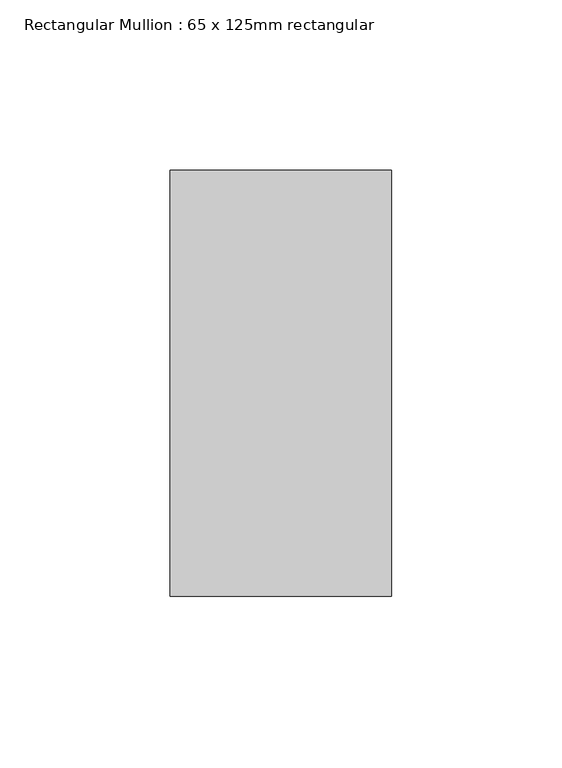
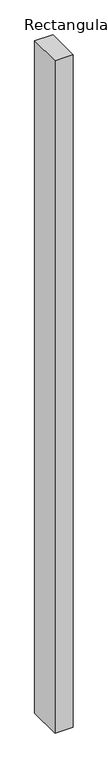
"""IFC4 building model written with IfcOpenShell, lengths in millimetres: member geometry, Rectangular Mullion : 65 x 125mm rectangular."""

from ifc_helpers import new_model, si_unit, frame, origin, place, context, project, spatial, polyline, outline, extrude, source, transform, mapped, element, save


def rectangular_mullion_65_x_125mm_rectangular_89386302(model_context):
    return source(origin(), model_context, "Body", "SweptSolid", [
        extrude(outline(polyline([(32.5, 62.5), (32.5, -62.5), (-32.5, -62.5), (-32.5, 62.5), (32.5, 62.5)])), frame((0.0, 0.0, -2550.0), z_axis=(0.0, 0.0, 1.0), x_axis=(1.0, 0.0, 0.0)), (0.0, 0.0, 1.0), 2550.0),
    ])


if __name__ == "__main__":
    model = new_model("IFC4")
    model_context = context("Model", 3, world=origin())
    ifc_project = project(units=[si_unit("LENGTHUNIT", "METRE", prefix="MILLI")], contexts=[model_context])
    site = spatial("IfcSite", under=ifc_project)
    building = spatial("IfcBuilding", under=site)
    placement = place(None, origin())
    rectangular_mullion_65_x_125mm_rectangular_shape = rectangular_mullion_65_x_125mm_rectangular_89386302(model_context)
    element("IfcMember", 1, ObjectType="Rectangular Mullion : 65 x 125mm rectangular", at=placement, inside=building, context=model_context, shape_type="MappedRepresentation", body=[
        mapped(rectangular_mullion_65_x_125mm_rectangular_shape, transform((0.0, 0.0, 0.0), x_axis=(1.0, 0.0, 0.0), y_axis=(0.0, 1.0, 0.0), z_axis=(0.0, 0.0, 1.0))),
    ])
    save(model, "model.ifc")

# Revit data of these elements
# Type "Rectangular Mullion : 65 x 125mm rectangular"
#   built-in parameter 1007304 = 0.410105 (stored number, unit not read)
#   built-in parameter 1007301 = 0.106627 (stored number, unit not read)
#   built-in parameter 1007300 = 0.106627 (stored number, unit not read)
# Element 1 (IfcMember, "Rectangular Mullion : 65 x 125mm rectangular")
#   Materials on its faces: "Aluminum"
# Materials
#   "Aluminum": class "Metal", colour RGB 244 245 246, transparency 0, Description = "Aluminum 6061", Cost = 0
